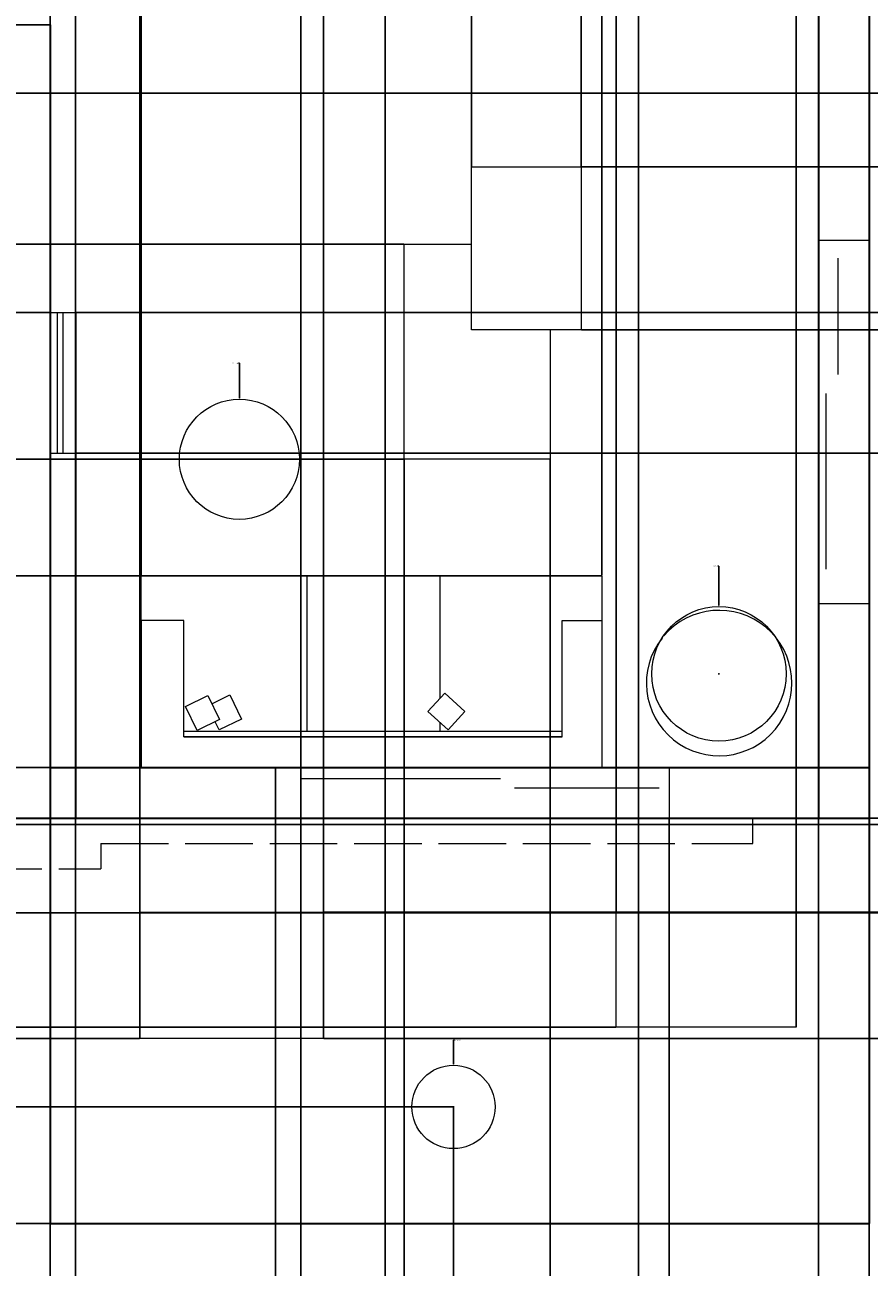
# Model space of a CAD drawing. Units: inches. Extents: x -47 to 496, y -43 to 706.
# Tile 3 of 6: x 209 to 359, y 123 to 344. Entities that reach past the tile are written whole.
import ezdxf

# ---------------------------------------------------------------- set-up
doc = ezdxf.new("R2010")
doc.units = ezdxf.units.IN
doc.linetypes.add('ACAD_ISO02W100', pattern=[15, 12, -3])
for name, color, linetype, lineweight in [('A-ANNO-DIMS', 2, 'Continuous', 18), ('A-ROOF-OVHD', 8, 'ACAD_ISO02W100', 18), ('FURNITURE', 3, 'Continuous', 18), ('WALL', 7, 'Continuous', 35), ('WINDOW', 1, 'Continuous', 18)]:
    doc.layers.add(name, color=color, linetype=linetype, lineweight=lineweight)
doc.styles.get("Standard").update_dxf_attribs({"font": 'arial.ttf'})
doc.dimstyles.get("Standard").update_dxf_attribs({"dimtxt": 0.18, "dimasz": 0.18, "dimexe": 0.18, "dimexo": 0.0625, "dimgap": 0.09, "dimtad": 0, "dimtih": 1, "dimtoh": 1, "dimdec": 4, "dimzin": 0, "dimdsep": 46, "dimtxsty": 'Standard', "dimcen": 0.09, "dimadec": 0, "dimazin": 0, "dimtfac": 1, "dimtdec": 4, "dimtofl": 0, "dimtmove": 0, "dimatfit": 3, "dimfxl": 1, "dimtolj": 1, "dimtzin": 0, "dimarcsym": 0})

# ---------------------------------------------------------------- blocks, each defined once
blk = doc.blocks.new('*D21')
at = {"layer": 'A-ANNO-DIMS', "color": 0, "lineweight": -2, "transparency": 16777216}
for p, q in [((213.95, 130.91), (213.95, -42.84)), ((359.45, 130.91), (359.45, -42.84)), ((214.13, -42.66), (286.32, -42.66)), ((359.27, -42.66), (287.09, -42.66))]:
    blk.add_line(p, q, dxfattribs=at)
at = {"layer": 'A-ANNO-DIMS', "color": 0, "transparency": 16777216}
for points in [[(214.13, -42.63), (214.13, -42.69), (213.95, -42.66)], [(359.27, -42.63), (359.27, -42.69), (359.45, -42.66)]]:
    blk.add_solid(points, dxfattribs=at)
at = {"layer": 'Defpoints', "color": 0, "transparency": 16777216}
for p in [(213.95, 130.97), (359.45, 130.97), (359.45, -42.66)]:
    blk.add_point(p, dxfattribs=at)
at = {"layer": 'A-ANNO-DIMS', "color": 0, "transparency": 16777216, "insert": (286.7, -42.66), "char_height": 0.18, "attachment_point": 5}
blk.add_mtext('\\A1;145.5', dxfattribs=at)
blk = doc.blocks.new('*D22')
at = {"layer": 'A-ANNO-DIMS', "color": 0, "lineweight": -2, "transparency": 16777216}
for p, q in [((229.88, 163.9), (229.88, 705.7)), ((230.06, 705.52), (245.73, 705.52)), ((262.33, 705.52), (246.66, 705.52)), ((262.51, 163.9), (262.51, 705.7))]:
    blk.add_line(p, q, dxfattribs=at)
at = {"layer": 'A-ANNO-DIMS', "color": 0, "transparency": 16777216}
for points in [[(230.06, 705.55), (230.06, 705.49), (229.88, 705.52)], [(262.33, 705.55), (262.33, 705.49), (262.51, 705.52)]]:
    blk.add_solid(points, dxfattribs=at)
at = {"layer": 'Defpoints', "color": 0, "transparency": 16777216}
for p in [(262.51, 705.52), (229.88, 163.83), (262.51, 163.83)]:
    blk.add_point(p, dxfattribs=at)
at = {"layer": 'A-ANNO-DIMS', "color": 0, "transparency": 16777216, "insert": (246.2, 705.52), "char_height": 0.18, "attachment_point": 5}
blk.add_mtext('\\A1;32.636', dxfattribs=at)
blk = doc.blocks.new('*D23')
at = {"layer": 'A-ANNO-DIMS', "color": 0, "lineweight": -2, "transparency": 16777216}
for p, q in [((262.58, 186.29), (496.14, 186.29)), ((495.96, 186.11), (495.96, 175.24)), ((495.96, 164.01), (495.96, 174.88)), ((262.58, 163.83), (496.14, 163.83))]:
    blk.add_line(p, q, dxfattribs=at)
at = {"layer": 'A-ANNO-DIMS', "color": 0, "transparency": 16777216}
for points in [[(495.93, 186.11), (495.99, 186.11), (495.96, 186.29)], [(495.93, 164.01), (495.99, 164.01), (495.96, 163.83)]]:
    blk.add_solid(points, dxfattribs=at)
at = {"layer": 'Defpoints', "color": 0, "transparency": 16777216}
for p in [(262.51, 186.29), (495.96, 186.29), (262.51, 163.83)]:
    blk.add_point(p, dxfattribs=at)
at = {"layer": 'A-ANNO-DIMS', "color": 0, "transparency": 16777216, "insert": (495.96, 175.06), "char_height": 0.18, "attachment_point": 5}
blk.add_mtext('\\A1;22.45', dxfattribs=at)
blk = doc.blocks.new('*D24')
at = {"layer": 'A-ANNO-DIMS', "color": 0, "lineweight": -2, "transparency": 16777216}
for p, q in [((314.53, 186.25), (314.53, 705.7)), ((314.71, 705.52), (330.12, 705.52)), ((346.32, 705.52), (330.91, 705.52)), ((346.5, 186.25), (346.5, 705.7))]:
    blk.add_line(p, q, dxfattribs=at)
at = {"layer": 'A-ANNO-DIMS', "color": 0, "transparency": 16777216}
for points in [[(314.71, 705.55), (314.71, 705.49), (314.53, 705.52)], [(346.32, 705.55), (346.32, 705.49), (346.5, 705.52)]]:
    blk.add_solid(points, dxfattribs=at)
at = {"layer": 'Defpoints', "color": 0, "transparency": 16777216}
for p in [(346.5, 705.52), (314.53, 186.18), (346.5, 186.18)]:
    blk.add_point(p, dxfattribs=at)
at = {"layer": 'A-ANNO-DIMS', "color": 0, "transparency": 16777216, "insert": (330.52, 705.52), "char_height": 0.18, "attachment_point": 5}
blk.add_mtext('\\A1;31.97', dxfattribs=at)
blk = doc.blocks.new('*D25')
at = {"layer": 'A-ANNO-DIMS', "color": 0, "lineweight": -2, "transparency": 16777216}
for p, q in [((314.47, 186.18), (-47.29, 186.18)), ((-47.11, 186), (-47.11, 176.21)), ((-47.11, 166.05), (-47.11, 175.84)), ((314.47, 165.87), (-47.29, 165.87))]:
    blk.add_line(p, q, dxfattribs=at)
at = {"layer": 'A-ANNO-DIMS', "color": 0, "transparency": 16777216}
for points in [[(-47.14, 186), (-47.08, 186), (-47.11, 186.18)], [(-47.14, 166.05), (-47.08, 166.05), (-47.11, 165.87)]]:
    blk.add_solid(points, dxfattribs=at)
at = {"layer": 'Defpoints', "color": 0, "transparency": 16777216}
for p in [(-47.11, 186.18), (314.53, 186.18), (314.53, 165.87)]:
    blk.add_point(p, dxfattribs=at)
at = {"layer": 'A-ANNO-DIMS', "color": 0, "transparency": 16777216, "insert": (-47.11, 176.03), "char_height": 0.18, "attachment_point": 5}
blk.add_mtext('\\A1;20.318', dxfattribs=at)
blk = doc.blocks.new('*D26')
at = {"layer": 'A-ANNO-DIMS', "color": 0, "lineweight": -2, "transparency": 16777216}
for p, q in [((213.95, 131.03), (213.95, 705.7)), ((214.13, 705.52), (221.46, 705.52)), ((229.7, 705.52), (222.37, 705.52)), ((229.88, 163.9), (229.88, 705.7))]:
    blk.add_line(p, q, dxfattribs=at)
at = {"layer": 'A-ANNO-DIMS', "color": 0, "transparency": 16777216}
for points in [[(214.13, 705.55), (214.13, 705.49), (213.95, 705.52)], [(229.7, 705.55), (229.7, 705.49), (229.88, 705.52)]]:
    blk.add_solid(points, dxfattribs=at)
at = {"layer": 'Defpoints', "color": 0, "transparency": 16777216}
for p in [(229.88, 705.52), (229.88, 163.83), (213.95, 130.97)]:
    blk.add_point(p, dxfattribs=at)
at = {"layer": 'A-ANNO-DIMS', "color": 0, "transparency": 16777216, "insert": (221.92, 705.52), "char_height": 0.18, "attachment_point": 5}
blk.add_mtext('\\A1;15.924', dxfattribs=at)
blk = doc.blocks.new('*D27')
at = {"layer": 'A-ANNO-DIMS', "color": 0, "lineweight": -2, "transparency": 16777216}
for p, q in [((229.82, 163.83), (-47.29, 163.83)), ((-47.11, 163.65), (-47.11, 147.58)), ((-47.11, 131.15), (-47.11, 147.22)), ((213.89, 130.97), (-47.29, 130.97))]:
    blk.add_line(p, q, dxfattribs=at)
at = {"layer": 'A-ANNO-DIMS', "color": 0, "transparency": 16777216}
for points in [[(-47.14, 163.65), (-47.08, 163.65), (-47.11, 163.83)], [(-47.14, 131.15), (-47.08, 131.15), (-47.11, 130.97)]]:
    blk.add_solid(points, dxfattribs=at)
at = {"layer": 'Defpoints', "color": 0, "transparency": 16777216}
for p in [(-47.11, 163.83), (229.88, 163.83), (213.95, 130.97)]:
    blk.add_point(p, dxfattribs=at)
at = {"layer": 'A-ANNO-DIMS', "color": 0, "transparency": 16777216, "insert": (-47.11, 147.4), "char_height": 0.18, "attachment_point": 5}
blk.add_mtext('\\A1;32.864', dxfattribs=at)
blk = doc.blocks.new('*D28')
at = {"layer": 'A-ANNO-DIMS', "color": 0, "lineweight": -2, "transparency": 16777216}
for p, q in [((346.5, 165.93), (346.5, 705.7)), ((346.68, 705.52), (352.52, 705.52)), ((359.27, 705.52), (353.43, 705.52)), ((359.45, 131.03), (359.45, 705.7))]:
    blk.add_line(p, q, dxfattribs=at)
at = {"layer": 'A-ANNO-DIMS', "color": 0, "transparency": 16777216}
for points in [[(346.68, 705.55), (346.68, 705.49), (346.5, 705.52)], [(359.27, 705.55), (359.27, 705.49), (359.45, 705.52)]]:
    blk.add_solid(points, dxfattribs=at)
at = {"layer": 'Defpoints', "color": 0, "transparency": 16777216}
for p in [(359.45, 705.52), (346.5, 165.87), (359.45, 130.97)]:
    blk.add_point(p, dxfattribs=at)
at = {"layer": 'A-ANNO-DIMS', "color": 0, "transparency": 16777216, "insert": (352.98, 705.52), "char_height": 0.18, "attachment_point": 5}
blk.add_mtext('\\A1;12.954', dxfattribs=at)
blk = doc.blocks.new('*D29')
at = {"layer": 'A-ANNO-DIMS', "color": 0, "lineweight": -2, "transparency": 16777216}
for p, q in [((359.52, 202.97), (496.14, 202.97)), ((495.96, 202.79), (495.96, 194.76)), ((495.96, 186.36), (495.96, 194.4)), ((346.56, 186.18), (496.14, 186.18))]:
    blk.add_line(p, q, dxfattribs=at)
at = {"layer": 'A-ANNO-DIMS', "color": 0, "transparency": 16777216}
for points in [[(495.93, 202.79), (495.99, 202.79), (495.96, 202.97)], [(495.93, 186.36), (495.99, 186.36), (495.96, 186.18)]]:
    blk.add_solid(points, dxfattribs=at)
at = {"layer": 'Defpoints', "color": 0, "transparency": 16777216}
for p in [(359.45, 202.97), (495.96, 202.97), (346.5, 186.18)]:
    blk.add_point(p, dxfattribs=at)
at = {"layer": 'A-ANNO-DIMS', "color": 0, "transparency": 16777216, "insert": (495.96, 194.58), "char_height": 0.18, "attachment_point": 5}
blk.add_mtext('\\A1;16.787', dxfattribs=at)
blk = doc.blocks.new('*D30')
at = {"layer": 'A-ANNO-DIMS', "color": 0, "lineweight": -2, "transparency": 16777216}
for p, q in [((285.61, 151.6), (285.61, -42.84)), ((213.95, 130.91), (213.95, -42.84)), ((214.13, -42.66), (249.39, -42.66)), ((285.43, -42.66), (250.18, -42.66))]:
    blk.add_line(p, q, dxfattribs=at)
at = {"layer": 'A-ANNO-DIMS', "color": 0, "transparency": 16777216}
for points in [[(214.13, -42.63), (214.13, -42.69), (213.95, -42.66)], [(285.43, -42.63), (285.43, -42.69), (285.61, -42.66)]]:
    blk.add_solid(points, dxfattribs=at)
at = {"layer": 'Defpoints', "color": 0, "transparency": 16777216}
for p in [(285.61, 151.67), (213.95, 130.97), (285.61, -42.66)]:
    blk.add_point(p, dxfattribs=at)
at = {"layer": 'A-ANNO-DIMS', "color": 0, "transparency": 16777216, "insert": (249.78, -42.66), "char_height": 0.18, "attachment_point": 5}
blk.add_mtext('\\A1;71.65', dxfattribs=at)
blk = doc.blocks.new('*D31')
at = {"layer": 'A-ANNO-DIMS', "color": 0, "lineweight": -2, "transparency": 16777216}
for p, q in [((285.55, 151.67), (-47.29, 151.67)), ((-47.11, 151.49), (-47.11, 141.5)), ((-47.11, 131.15), (-47.11, 141.14)), ((359.39, 130.97), (-47.29, 130.97))]:
    blk.add_line(p, q, dxfattribs=at)
at = {"layer": 'A-ANNO-DIMS', "color": 0, "transparency": 16777216}
for points in [[(-47.14, 151.49), (-47.08, 151.49), (-47.11, 151.67)], [(-47.14, 131.15), (-47.08, 131.15), (-47.11, 130.97)]]:
    blk.add_solid(points, dxfattribs=at)
at = {"layer": 'Defpoints', "color": 0, "transparency": 16777216}
for p in [(285.61, 151.67), (-47.11, 130.97), (359.45, 130.97)]:
    blk.add_point(p, dxfattribs=at)
at = {"layer": 'A-ANNO-DIMS', "color": 0, "transparency": 16777216, "insert": (-47.11, 141.32), "char_height": 0.18, "attachment_point": 5}
blk.add_mtext('\\A1;20.695', dxfattribs=at)
blk = doc.blocks.new('*D35')
at = {"layer": 'A-ANNO-DIMS', "color": 0, "lineweight": -2, "transparency": 16777216}
for p, q in [((218.45, 484.91), (218.45, -42.84)), ((350.45, 480.41), (350.45, -42.84)), ((218.63, -42.66), (284.18, -42.66)), ((350.27, -42.66), (284.73, -42.66))]:
    blk.add_line(p, q, dxfattribs=at)
at = {"layer": 'A-ANNO-DIMS', "color": 0, "transparency": 16777216}
for points in [[(218.63, -42.63), (218.63, -42.69), (218.45, -42.66)], [(350.27, -42.63), (350.27, -42.69), (350.45, -42.66)]]:
    blk.add_solid(points, dxfattribs=at)
at = {"layer": 'Defpoints', "color": 0, "transparency": 16777216}
for p in [(218.45, 484.97), (350.45, 480.47), (350.45, -42.66)]:
    blk.add_point(p, dxfattribs=at)
at = {"layer": 'A-ANNO-DIMS', "color": 0, "transparency": 16777216, "insert": (284.45, -42.66), "char_height": 0.18, "attachment_point": 5}
blk.add_mtext('\\A1;132', dxfattribs=at)
blk = doc.blocks.new('*D51')
at = {"layer": 'A-ANNO-DIMS', "color": 0, "lineweight": -2, "transparency": 16777216}
for p, q in [((218.45, 621.91), (218.45, -42.84)), ((258.46, 619.91), (258.46, -42.84)), ((218.63, -42.66), (238.08, -42.66)), ((258.28, -42.66), (238.84, -42.66))]:
    blk.add_line(p, q, dxfattribs=at)
at = {"layer": 'A-ANNO-DIMS', "color": 0, "transparency": 16777216}
for points in [[(218.63, -42.63), (218.63, -42.69), (218.45, -42.66)], [(258.28, -42.63), (258.28, -42.69), (258.46, -42.66)]]:
    blk.add_solid(points, dxfattribs=at)
at = {"layer": 'Defpoints', "color": 0, "transparency": 16777216}
for p in [(218.45, 621.97), (258.46, 619.97), (258.46, -42.66)]:
    blk.add_point(p, dxfattribs=at)
at = {"layer": 'A-ANNO-DIMS', "color": 0, "transparency": 16777216, "insert": (238.46, -42.66), "char_height": 0.18, "attachment_point": 5}
blk.add_mtext('\\A1;40.01', dxfattribs=at)
blk = doc.blocks.new('*D54')
at = {"layer": 'A-ANNO-DIMS', "color": 0, "lineweight": -2, "transparency": 16777216}
for p, q in [((273.48, 348.41), (273.48, -42.84)), ((350.45, 348.41), (350.45, -42.84)), ((273.66, -42.66), (311.57, -42.66)), ((350.27, -42.66), (312.36, -42.66))]:
    blk.add_line(p, q, dxfattribs=at)
at = {"layer": 'A-ANNO-DIMS', "color": 0, "transparency": 16777216}
for points in [[(273.66, -42.63), (273.66, -42.69), (273.48, -42.66)], [(350.27, -42.63), (350.27, -42.69), (350.45, -42.66)]]:
    blk.add_solid(points, dxfattribs=at)
at = {"layer": 'Defpoints', "color": 0, "transparency": 16777216}
for p in [(273.48, 348.47), (350.45, 348.47), (350.45, -42.66)]:
    blk.add_point(p, dxfattribs=at)
at = {"layer": 'A-ANNO-DIMS', "color": 0, "transparency": 16777216, "insert": (311.97, -42.66), "char_height": 0.18, "attachment_point": 5}
blk.add_mtext('\\A1;76.97', dxfattribs=at)
blk = doc.blocks.new('*D59')
at = {"layer": 'A-ANNO-DIMS', "color": 0, "lineweight": -2, "transparency": 16777216}
for p, q in [((318.48, 390.41), (318.48, -42.84)), ((350.45, 390.41), (350.45, -42.84)), ((318.66, -42.66), (334, -42.66)), ((350.27, -42.66), (334.93, -42.66))]:
    blk.add_line(p, q, dxfattribs=at)
at = {"layer": 'A-ANNO-DIMS', "color": 0, "transparency": 16777216}
for points in [[(318.66, -42.63), (318.66, -42.69), (318.48, -42.66)], [(350.27, -42.63), (350.27, -42.69), (350.45, -42.66)]]:
    blk.add_solid(points, dxfattribs=at)
at = {"layer": 'Defpoints', "color": 0, "transparency": 16777216}
for p in [(318.48, 390.47), (350.45, 390.47), (350.45, -42.66)]:
    blk.add_point(p, dxfattribs=at)
at = {"layer": 'A-ANNO-DIMS', "color": 0, "transparency": 16777216, "insert": (334.47, -42.66), "char_height": 0.18, "attachment_point": 5}
blk.add_mtext('\\A1;31.975', dxfattribs=at)
blk = doc.blocks.new('*D64')
at = {"layer": 'A-ANNO-DIMS', "color": 0, "lineweight": -2, "transparency": 16777216}
for p, q in [((158.02, 343.91), (158.02, -42.84)), ((218.45, 343.91), (218.45, -42.84)), ((158.2, -42.66), (187.84, -42.66)), ((218.27, -42.66), (188.63, -42.66))]:
    blk.add_line(p, q, dxfattribs=at)
at = {"layer": 'A-ANNO-DIMS', "color": 0, "transparency": 16777216}
for points in [[(158.2, -42.63), (158.2, -42.69), (158.02, -42.66)], [(218.27, -42.63), (218.27, -42.69), (218.45, -42.66)]]:
    blk.add_solid(points, dxfattribs=at)
at = {"layer": 'Defpoints', "color": 0, "transparency": 16777216}
for p in [(158.02, 343.97), (218.45, 343.97), (218.45, -42.66)]:
    blk.add_point(p, dxfattribs=at)
at = {"layer": 'A-ANNO-DIMS', "color": 0, "transparency": 16777216, "insert": (188.24, -42.66), "char_height": 0.18, "attachment_point": 5}
blk.add_mtext('\\A1;60.43', dxfattribs=at)
blk = doc.blocks.new('*D65')
at = {"layer": 'A-ANNO-DIMS', "color": 0, "lineweight": -2, "transparency": 16777216}
for p, q in [((218.45, 348.41), (218.45, -42.84)), ((273.48, 348.41), (273.48, -42.84)), ((218.63, -42.66), (245.57, -42.66)), ((273.3, -42.66), (246.36, -42.66))]:
    blk.add_line(p, q, dxfattribs=at)
at = {"layer": 'A-ANNO-DIMS', "color": 0, "transparency": 16777216}
for points in [[(218.63, -42.63), (218.63, -42.69), (218.45, -42.66)], [(273.3, -42.63), (273.3, -42.69), (273.48, -42.66)]]:
    blk.add_solid(points, dxfattribs=at)
at = {"layer": 'Defpoints', "color": 0, "transparency": 16777216}
for p in [(218.45, 348.47), (273.48, 348.47), (273.48, -42.66)]:
    blk.add_point(p, dxfattribs=at)
at = {"layer": 'A-ANNO-DIMS', "color": 0, "transparency": 16777216, "insert": (245.97, -42.66), "char_height": 0.18, "attachment_point": 5}
blk.add_mtext('\\A1;55.03', dxfattribs=at)
blk = doc.blocks.new('*D73')
at = {"layer": 'A-ANNO-DIMS', "color": 0, "lineweight": -2, "transparency": 16777216}
for p, q in [((213.95, 211.91), (213.95, -42.84)), ((195.95, 202.91), (195.95, -42.84)), ((196.13, -42.66), (204.74, -42.66)), ((213.77, -42.66), (205.17, -42.66))]:
    blk.add_line(p, q, dxfattribs=at)
at = {"layer": 'A-ANNO-DIMS', "color": 0, "transparency": 16777216}
for points in [[(196.13, -42.63), (196.13, -42.69), (195.95, -42.66)], [(213.77, -42.63), (213.77, -42.69), (213.95, -42.66)]]:
    blk.add_solid(points, dxfattribs=at)
at = {"layer": 'Defpoints', "color": 0, "transparency": 16777216}
for p in [(213.95, 211.97), (195.95, 202.97), (213.95, -42.66)]:
    blk.add_point(p, dxfattribs=at)
at = {"layer": 'A-ANNO-DIMS', "color": 0, "transparency": 16777216, "insert": (204.95, -42.66), "char_height": 0.18, "attachment_point": 5}
blk.add_mtext('\\A1;18', dxfattribs=at)
blk = doc.blocks.new('*D74')
at = {"layer": 'A-ANNO-DIMS', "color": 0, "lineweight": -2, "transparency": 16777216}
for p, q in [((213.95, 211.91), (213.95, -42.84)), ((254, 211.91), (254, -42.84)), ((214.13, -42.66), (233.58, -42.66)), ((253.82, -42.66), (234.38, -42.66))]:
    blk.add_line(p, q, dxfattribs=at)
at = {"layer": 'A-ANNO-DIMS', "color": 0, "transparency": 16777216}
for points in [[(214.13, -42.63), (214.13, -42.69), (213.95, -42.66)], [(253.82, -42.63), (253.82, -42.69), (254, -42.66)]]:
    blk.add_solid(points, dxfattribs=at)
at = {"layer": 'Defpoints', "color": 0, "transparency": 16777216}
for p in [(213.95, 211.97), (254, 211.97), (254, -42.66)]:
    blk.add_point(p, dxfattribs=at)
at = {"layer": 'A-ANNO-DIMS', "color": 0, "transparency": 16777216, "insert": (233.98, -42.66), "char_height": 0.18, "attachment_point": 5}
blk.add_mtext('\\A1;40.05', dxfattribs=at)
blk = doc.blocks.new('*D75')
at = {"layer": 'A-ANNO-DIMS', "color": 0, "lineweight": -2, "transparency": 16777216}
for p, q in [((254, 202.91), (254, -42.84)), ((323.91, 202.91), (323.91, -42.84)), ((254.18, -42.66), (288.58, -42.66)), ((323.73, -42.66), (289.33, -42.66))]:
    blk.add_line(p, q, dxfattribs=at)
at = {"layer": 'A-ANNO-DIMS', "color": 0, "transparency": 16777216}
for points in [[(254.18, -42.63), (254.18, -42.69), (254, -42.66)], [(323.73, -42.63), (323.73, -42.69), (323.91, -42.66)]]:
    blk.add_solid(points, dxfattribs=at)
at = {"layer": 'Defpoints', "color": 0, "transparency": 16777216}
for p in [(254, 202.97), (323.91, 202.97), (323.91, -42.66)]:
    blk.add_point(p, dxfattribs=at)
at = {"layer": 'A-ANNO-DIMS', "color": 0, "transparency": 16777216, "insert": (288.96, -42.66), "char_height": 0.18, "attachment_point": 5}
blk.add_mtext('\\A1;69.91', dxfattribs=at)
blk = doc.blocks.new('*D78')
at = {"layer": 'A-ANNO-DIMS', "color": 0, "lineweight": -2, "transparency": 16777216}
for p, q in [((230.13, 246.14), (230.13, 705.7)), ((230.31, 705.52), (270.64, 705.52)), ((311.77, 705.52), (271.43, 705.52)), ((311.95, 246.14), (311.95, 705.7))]:
    blk.add_line(p, q, dxfattribs=at)
at = {"layer": 'A-ANNO-DIMS', "color": 0, "transparency": 16777216}
for points in [[(230.31, 705.55), (230.31, 705.49), (230.13, 705.52)], [(311.77, 705.55), (311.77, 705.49), (311.95, 705.52)]]:
    blk.add_solid(points, dxfattribs=at)
at = {"layer": 'Defpoints', "color": 0, "transparency": 16777216}
for p in [(311.95, 705.52), (230.13, 246.07), (311.95, 246.07)]:
    blk.add_point(p, dxfattribs=at)
at = {"layer": 'A-ANNO-DIMS', "color": 0, "transparency": 16777216, "insert": (271.04, 705.52), "char_height": 0.18, "attachment_point": 5}
blk.add_mtext('\\A1;81.82', dxfattribs=at)
blk = doc.blocks.new('*D79')
at = {"layer": 'A-ANNO-DIMS', "color": 0, "lineweight": -2, "transparency": 16777216}
for p, q in [((311.88, 246.07), (-47.29, 246.07)), ((-47.11, 245.89), (-47.11, 229.2)), ((-47.11, 212.15), (-47.11, 228.84)), ((311.88, 211.97), (-47.29, 211.97))]:
    blk.add_line(p, q, dxfattribs=at)
at = {"layer": 'A-ANNO-DIMS', "color": 0, "transparency": 16777216}
for points in [[(-47.14, 245.89), (-47.08, 245.89), (-47.11, 246.07)], [(-47.14, 212.15), (-47.08, 212.15), (-47.11, 211.97)]]:
    blk.add_solid(points, dxfattribs=at)
at = {"layer": 'Defpoints', "color": 0, "transparency": 16777216}
for p in [(-47.11, 246.07), (311.95, 246.07), (311.95, 211.97)]:
    blk.add_point(p, dxfattribs=at)
at = {"layer": 'A-ANNO-DIMS', "color": 0, "transparency": 16777216, "insert": (-47.11, 229.02), "char_height": 0.18, "attachment_point": 5}
blk.add_mtext('\\A1;34.103', dxfattribs=at)
blk = doc.blocks.new('*D80')
at = {"layer": 'A-ANNO-DIMS', "color": 0, "lineweight": -2, "transparency": 16777216}
for p, q in [((218.52, 292.83), (496.14, 292.83)), ((495.96, 292.65), (495.96, 280.53)), ((495.96, 268.06), (495.96, 280.17)), ((218.52, 267.88), (496.14, 267.88))]:
    blk.add_line(p, q, dxfattribs=at)
at = {"layer": 'A-ANNO-DIMS', "color": 0, "transparency": 16777216}
for points in [[(495.93, 292.65), (495.99, 292.65), (495.96, 292.83)], [(495.93, 268.06), (495.99, 268.06), (495.96, 267.88)]]:
    blk.add_solid(points, dxfattribs=at)
at = {"layer": 'Defpoints', "color": 0, "transparency": 16777216}
for p in [(218.45, 292.83), (495.96, 292.83), (218.45, 267.88)]:
    blk.add_point(p, dxfattribs=at)
at = {"layer": 'A-ANNO-DIMS', "color": 0, "transparency": 16777216, "insert": (495.96, 280.35), "char_height": 0.18, "attachment_point": 5}
blk.add_mtext('\\A1;24.946', dxfattribs=at)
blk = doc.blocks.new('*D81')
at = {"layer": 'A-ANNO-DIMS', "color": 0, "lineweight": -2, "transparency": 16777216}
for p, q in [((213.89, 343.97), (-47.29, 343.97)), ((-47.11, 343.79), (-47.11, 318.58)), ((-47.11, 293.01), (-47.11, 318.22)), ((213.89, 292.83), (-47.29, 292.83))]:
    blk.add_line(p, q, dxfattribs=at)
at = {"layer": 'A-ANNO-DIMS', "color": 0, "transparency": 16777216}
for points in [[(-47.14, 343.79), (-47.08, 343.79), (-47.11, 343.97)], [(-47.14, 293.01), (-47.08, 293.01), (-47.11, 292.83)]]:
    blk.add_solid(points, dxfattribs=at)
at = {"layer": 'Defpoints', "color": 0, "transparency": 16777216}
for p in [(-47.11, 343.97), (213.95, 343.97), (213.95, 292.83)]:
    blk.add_point(p, dxfattribs=at)
at = {"layer": 'A-ANNO-DIMS', "color": 0, "transparency": 16777216, "insert": (-47.11, 318.4), "char_height": 0.18, "attachment_point": 5}
blk.add_mtext('\\A1;51.15', dxfattribs=at)
blk = doc.blocks.new('*D82')
at = {"layer": 'A-ANNO-DIMS', "color": 0, "lineweight": -2, "transparency": 16777216}
for p, q in [((108.88, 331.8), (496.14, 331.8)), ((495.96, 331.62), (495.96, 267)), ((495.96, 202.02), (495.96, 266.64)), ((131.48, 201.84), (496.14, 201.84))]:
    blk.add_line(p, q, dxfattribs=at)
at = {"layer": 'A-ANNO-DIMS', "color": 0, "transparency": 16777216}
for points in [[(495.93, 331.62), (495.99, 331.62), (495.96, 331.8)], [(495.93, 202.02), (495.99, 202.02), (495.96, 201.84)]]:
    blk.add_solid(points, dxfattribs=at)
at = {"layer": 'Defpoints', "color": 0, "transparency": 16777216}
for p in [(108.82, 331.8), (131.41, 201.84), (495.96, 201.84)]:
    blk.add_point(p, dxfattribs=at)
at = {"layer": 'A-ANNO-DIMS', "color": 0, "transparency": 16777216, "insert": (495.96, 266.82), "char_height": 0.18, "attachment_point": 5}
blk.add_mtext('\\A1;129.95', dxfattribs=at)
blk = doc.blocks.new('*D84')
at = {"layer": 'A-ANNO-DIMS', "color": 0, "lineweight": -2, "transparency": 16777216}
for p, q in [((276.84, 266.72), (276.84, -42.84)), ((302.79, 266.72), (302.79, -42.84)), ((277.02, -42.66), (289.42, -42.66)), ((302.61, -42.66), (290.21, -42.66))]:
    blk.add_line(p, q, dxfattribs=at)
at = {"layer": 'A-ANNO-DIMS', "color": 0, "transparency": 16777216}
for points in [[(277.02, -42.63), (277.02, -42.69), (276.84, -42.66)], [(302.61, -42.63), (302.61, -42.69), (302.79, -42.66)]]:
    blk.add_solid(points, dxfattribs=at)
at = {"layer": 'Defpoints', "color": 0, "transparency": 16777216}
for p in [(276.84, 266.78), (302.79, 266.78), (302.79, -42.66)]:
    blk.add_point(p, dxfattribs=at)
at = {"layer": 'A-ANNO-DIMS', "color": 0, "transparency": 16777216, "insert": (289.82, -42.66), "char_height": 0.18, "attachment_point": 5}
blk.add_mtext('\\A1;25.95', dxfattribs=at)
blk = doc.blocks.new('*D85')
at = {"layer": 'A-ANNO-DIMS', "color": 0, "lineweight": -2, "transparency": 16777216}
for p, q in [((276.78, 305.01), (-47.29, 305.01)), ((-47.11, 304.83), (-47.11, 286.08)), ((-47.11, 266.96), (-47.11, 285.71)), ((276.78, 266.78), (-47.29, 266.78))]:
    blk.add_line(p, q, dxfattribs=at)
at = {"layer": 'A-ANNO-DIMS', "color": 0, "transparency": 16777216}
for points in [[(-47.14, 304.83), (-47.08, 304.83), (-47.11, 305.01)], [(-47.14, 266.96), (-47.08, 266.96), (-47.11, 266.78)]]:
    blk.add_solid(points, dxfattribs=at)
at = {"layer": 'Defpoints', "color": 0, "transparency": 16777216}
for p in [(-47.11, 305.01), (276.84, 305.01), (276.84, 266.78)]:
    blk.add_point(p, dxfattribs=at)
at = {"layer": 'A-ANNO-DIMS', "color": 0, "transparency": 16777216, "insert": (-47.11, 285.9), "char_height": 0.18, "attachment_point": 5}
blk.add_mtext('\\A1;38.22', dxfattribs=at)
blk = doc.blocks.new('*D86')
at = {"layer": 'A-ANNO-DIMS', "color": 0, "lineweight": -2, "transparency": 16777216}
for p, q in [((288.82, 318.79), (288.82, 705.7)), ((289, 705.52), (298.16, 705.52)), ((308.09, 705.52), (298.93, 705.52)), ((308.27, 318.79), (308.27, 705.7))]:
    blk.add_line(p, q, dxfattribs=at)
at = {"layer": 'A-ANNO-DIMS', "color": 0, "transparency": 16777216}
for points in [[(289, 705.55), (289, 705.49), (288.82, 705.52)], [(308.09, 705.55), (308.09, 705.49), (308.27, 705.52)]]:
    blk.add_solid(points, dxfattribs=at)
at = {"layer": 'Defpoints', "color": 0, "transparency": 16777216}
for p in [(308.27, 705.52), (288.82, 318.72), (308.27, 318.72)]:
    blk.add_point(p, dxfattribs=at)
at = {"layer": 'A-ANNO-DIMS', "color": 0, "transparency": 16777216, "insert": (298.54, 705.52), "char_height": 0.18, "attachment_point": 5}
blk.add_mtext('\\A1;19.45', dxfattribs=at)
blk = doc.blocks.new('*D87')
at = {"layer": 'A-ANNO-DIMS', "color": 0, "lineweight": -2, "transparency": 16777216}
for p, q in [((308.33, 318.72), (496.14, 318.72)), ((495.96, 318.54), (495.96, 304.44)), ((495.96, 289.97), (495.96, 304.07)), ((308.33, 289.79), (496.14, 289.79))]:
    blk.add_line(p, q, dxfattribs=at)
at = {"layer": 'A-ANNO-DIMS', "color": 0, "transparency": 16777216}
for points in [[(495.93, 318.54), (495.99, 318.54), (495.96, 318.72)], [(495.93, 289.97), (495.99, 289.97), (495.96, 289.79)]]:
    blk.add_solid(points, dxfattribs=at)
at = {"layer": 'Defpoints', "color": 0, "transparency": 16777216}
for p in [(308.27, 318.72), (495.96, 318.72), (308.27, 289.79)]:
    blk.add_point(p, dxfattribs=at)
at = {"layer": 'A-ANNO-DIMS', "color": 0, "transparency": 16777216, "insert": (495.96, 304.26), "char_height": 0.18, "attachment_point": 5}
blk.add_mtext('\\A1;28.94', dxfattribs=at)
blk = doc.blocks.new('*D88')
at = {"layer": 'A-ANNO-DIMS', "color": 0, "lineweight": -2, "transparency": 16777216}
for p, q in [((285.79, 163.51), (285.61, 163.51)), ((285.61, 163.51), (285.61, 159.25)), ((285.52, 151.67), (285.7, 151.67)), ((285.61, 151.58), (285.61, 151.76))]:
    blk.add_line(p, q, dxfattribs=at)
at = {"layer": 'A-ANNO-DIMS', "color": 0, "transparency": 16777216}
blk.add_solid([(285.58, 159.25), (285.64, 159.25), (285.61, 159.07)], dxfattribs=at)
at = {"layer": 'Defpoints', "color": 0, "transparency": 16777216}
for p in [(285.61, 159.07), (285.61, 144.26)]:
    blk.add_point(p, dxfattribs=at)
at = {"layer": 'A-ANNO-DIMS', "color": 0, "transparency": 16777216, "insert": (286.35, 163.51), "char_height": 0.18, "attachment_point": 5}
blk.add_mtext('\\A1;∅14.807', dxfattribs=at)
blk = doc.blocks.new('*D90')
at = {"layer": 'A-ANNO-DIMS', "color": 0, "lineweight": -2, "transparency": 16777216}
for p, q in [((332.59, 247.76), (332.77, 247.76)), ((332.77, 247.76), (332.77, 240.76)), ((332.68, 228.63), (332.86, 228.63)), ((332.77, 228.54), (332.77, 228.72))]:
    blk.add_line(p, q, dxfattribs=at)
at = {"layer": 'A-ANNO-DIMS', "color": 0, "transparency": 16777216}
blk.add_solid([(332.8, 240.76), (332.74, 240.76), (332.77, 240.58)], dxfattribs=at)
at = {"layer": 'Defpoints', "color": 0, "transparency": 16777216}
for p in [(332.77, 240.58), (332.77, 216.68)]:
    blk.add_point(p, dxfattribs=at)
at = {"layer": 'A-ANNO-DIMS', "color": 0, "transparency": 16777216, "insert": (332.12, 247.76), "char_height": 0.18, "attachment_point": 5}
blk.add_mtext('\\A1;∅23.91', dxfattribs=at)
blk = doc.blocks.new('*D91')
at = {"layer": 'A-ANNO-DIMS', "color": 0, "lineweight": -2, "transparency": 16777216}
for p, q in [((247.4, 283.85), (247.58, 283.85)), ((247.58, 283.85), (247.58, 277.62)), ((247.49, 266.77), (247.67, 266.77)), ((247.58, 266.68), (247.58, 266.86))]:
    blk.add_line(p, q, dxfattribs=at)
at = {"layer": 'A-ANNO-DIMS', "color": 0, "transparency": 16777216}
blk.add_solid([(247.61, 277.62), (247.55, 277.62), (247.58, 277.44)], dxfattribs=at)
at = {"layer": 'Defpoints', "color": 0, "transparency": 16777216}
for p in [(247.58, 277.44), (247.58, 256.09)]:
    blk.add_point(p, dxfattribs=at)
at = {"layer": 'A-ANNO-DIMS', "color": 0, "transparency": 16777216, "insert": (246.84, 283.85), "char_height": 0.18, "attachment_point": 5}
blk.add_mtext('\\A1;∅21.354', dxfattribs=at)

msp = doc.modelspace()

# ---------------------------------------------------------------- linework, layer by layer
at = {"layer": 'A-ROOF-OVHD'}
for p, q in [((338.7999, 198.4711), (338.7999, 202.9711)), ((222.9545, 198.4711), (338.7999, 198.4711)), ((222.9545, 198.4711), (222.9545, 193.9711)), ((170.4932, 193.9711), (222.9545, 193.9711))]:
    msp.add_line(p, q, dxfattribs=at)
at = {"layer": 'FURNITURE'}
for p, q in [((259.5909, 218.421), (259.5909, 246.0745)), ((283.2401, 224.2901), (283.2401, 246.0745)), ((283.2401, 218.421), (283.2401, 219.9332))]:
    msp.add_line(p, q, dxfattribs=at)
for points in [[(288.8165, 318.7246), (308.2664, 318.7246), (308.2664, 289.7875), (288.8165, 289.7875)], [(237.9876, 222.8252), (241.971, 224.7682), (244.0536, 220.4987), (240.0702, 218.5557)], [(284.6398, 218.6567), (281.0709, 221.9114), (284.0659, 225.1956), (287.6349, 221.9409)], [(229.8783, 186.2855), (262.5138, 186.2855), (262.5138, 163.8346), (229.8783, 163.8346)], [(314.5329, 186.184), (346.5, 186.184), (346.5, 165.8664), (314.5329, 165.8664)]]:
    msp.add_lwpolyline(points, close=True, dxfattribs=at)
for points in [[(302.7925, 289.7875), (302.7925, 266.7848), (276.8411, 266.7848), (276.8411, 305.006), (288.8165, 305.006)], [(230.1291, 217.421), (230.1291, 246.0745), (311.9452, 246.0745), (311.9452, 217.421)], [(237.7272, 217.421), (237.7272, 238.1389), (230.1291, 238.1389), (230.1291, 211.9711), (237.7272, 211.9711)], [(304.9418, 217.421), (304.9418, 238.1389), (311.9452, 238.1389), (311.9452, 211.9711), (304.9418, 211.9711)], [(242.6823, 223.31), (245.8862, 224.8728), (247.9687, 220.6032), (243.9853, 218.6603), (243.2741, 220.1185)], [(311.9452, 217.421), (311.9452, 211.9711), (230.1291, 211.9711), (230.1291, 217.421)], [(237.7272, 218.421), (304.9418, 218.421)], [(237.7272, 217.421), (304.9418, 217.421)], [(304.9418, 217.421), (237.7272, 217.421)]]:
    msp.add_lwpolyline(points, dxfattribs=at)
for centre, radius in [((247.5772, 266.7661), 10.6769), ((332.7731, 228.6297), 11.9539), ((285.6085, 151.6661), 7.4034)]:
    msp.add_circle(centre, radius, dxfattribs=at)
msp.add_arc((332.8044, 226.9925), 12.9245, 141.764596, 139.573954, dxfattribs=at)
at = {"layer": 'WALL'}
for p, q in [((350.4545, 635.4711), (350.4545, 202.9711)), ((359.4545, 635.4711), (359.4545, 130.9711)), ((213.9545, 343.9711), (213.9545, 130.9711)), ((218.4545, 292.8257), (218.4545, 202.9711)), ((213.9545, 211.9711), (359.4545, 211.9711)), ((195.9545, 202.9711), (359.4545, 202.9711)), ((213.9545, 130.9711), (359.4545, 130.9711))]:
    msp.add_line(p, q, dxfattribs=at)
at = {"layer": 'WINDOW'}
for p, q in [((350.4545, 305.6843), (359.4545, 305.6843)), ((353.9691, 281.8522), (353.9691, 302.4765)), ((213.9545, 292.8257), (218.4545, 292.8257)), ((215.1987, 292.8257), (215.1987, 267.8798)), ((216.2045, 292.8257), (216.2045, 267.8798)), ((351.7782, 278.4445), (351.7782, 247.253)), ((213.9545, 267.8798), (218.4545, 267.8798)), ((350.4545, 241.1376), (359.4545, 241.1376)), ((254.0024, 211.9711), (254.0024, 202.9711)), ((323.9122, 211.9711), (323.9122, 202.9711)), ((258.6824, 210.0344), (293.9852, 210.0344)), ((296.4181, 208.3979), (322.1258, 208.3979))]:
    msp.add_line(p, q, dxfattribs=at)

# ---------------------------------------------------------------- dimensions: what is measured, and where the dimension line sits
at = {"layer": 'A-ANNO-DIMS'}
for base, p1, p2, override, picture, middle in [((229.8783, 705.5211), (213.9545, 130.9711), (229.8783, 163.8346), {"dimdec": 3, "dimlfac": 1, "dimrnd": 0, "dimzin": 0, "dimdsep": 46, "dimlunit": 2}, '*D26', (221.9164, 705.5211)), ((262.51385, 705.52106), (229.87829, 163.83464), (262.51385, 163.83464), {"dimdec": 3, "dimlfac": 1, "dimrnd": 0, "dimzin": 0, "dimdsep": 46, "dimlunit": 2}, '*D22', (246.19607, 705.52106)), ((311.9452, 705.5211), (230.1291, 246.0745), (311.9452, 246.0745), {"dimdec": 2, "dimlfac": 1, "dimrnd": 0, "dimzin": 0, "dimdsep": 46, "dimlunit": 2}, '*D78', (271.0372, 705.5211)), ((308.2664, 705.5211), (288.8165, 318.7246), (308.2664, 318.7246), {"dimdec": 2, "dimlfac": 1, "dimrnd": 0, "dimzin": 0, "dimdsep": 46, "dimlunit": 2}, '*D86', (298.5415, 705.5211)), ((346.5, 705.5211), (314.5329, 186.184), (346.5, 186.184), {"dimdec": 2, "dimlfac": 1, "dimrnd": 0, "dimzin": 0, "dimdsep": 46, "dimlunit": 2}, '*D24', (330.5165, 705.5211)), ((359.45448, 705.52106), (346.5, 165.86638), (359.45448, 130.97106), {"dimdec": 3, "dimlfac": 1, "dimrnd": 0, "dimzin": 0, "dimdsep": 46, "dimlunit": 2}, '*D28', (352.97724, 705.52106)), ((258.4633, -42.6632), (218.4545, 621.9711), (258.4633, 619.9711), {"dimdec": 2, "dimlfac": 1, "dimrnd": 0, "dimzin": 0, "dimdsep": 46, "dimlunit": 2}, '*D51', (238.4589, -42.6632)), ((350.4545, -42.6632), (218.4545, 484.9711), (350.4545, 480.4711), {"dimdec": 0, "dimlfac": 1, "dimrnd": 0, "dimzin": 0, "dimdsep": 46, "dimlunit": 2}, '*D35', (284.4545, -42.6632)), ((350.4545, -42.6632), (318.4798, 390.4711), (350.4545, 390.4711), {"dimdec": 3, "dimlfac": 1, "dimrnd": 0, "dimzin": 0, "dimdsep": 46, "dimlunit": 2}, '*D59', (334.4671, -42.6632)), ((273.4798, -42.6632), (218.4545, 348.4711), (273.4798, 348.4711), {"dimdec": 2, "dimlfac": 1, "dimrnd": 0, "dimzin": 0, "dimdsep": 46, "dimlunit": 2}, '*D65', (245.9671, -42.6632)), ((350.4545, -42.6632), (273.4798, 348.4711), (350.4545, 348.4711), {"dimdec": 2, "dimlfac": 1, "dimrnd": 0, "dimzin": 0, "dimdsep": 46, "dimlunit": 2}, '*D54', (311.9671, -42.6632)), ((218.4545, -42.6632), (158.0229, 343.9711), (218.4545, 343.9711), {"dimdec": 2, "dimlfac": 1, "dimrnd": 0, "dimzin": 0, "dimdsep": 46, "dimlunit": 2}, '*D64', (188.2387, -42.6632)), ((302.7925, -42.6632), (276.8411, 266.7848), (302.7925, 266.7848), {"dimdec": 2, "dimlfac": 1, "dimrnd": 0, "dimzin": 0, "dimdsep": 46, "dimlunit": 2}, '*D84', (289.8168, -42.6632)), ((213.9545, -42.6632), (195.9545, 202.9711), (213.9545, 211.9711), {"dimdec": 0, "dimlfac": 1, "dimrnd": 0, "dimzin": 0, "dimdsep": 46, "dimlunit": 2}, '*D73', (204.9545, -42.6632)), ((254.0024, -42.6632), (213.9545, 211.9711), (254.0024, 211.9711), {"dimdec": 2, "dimlfac": 1, "dimrnd": 0, "dimzin": 0, "dimdsep": 46, "dimlunit": 2}, '*D74', (233.9785, -42.6632)), ((323.9122, -42.6632), (254.0024, 202.9711), (323.9122, 202.9711), {"dimdec": 2, "dimlfac": 1, "dimrnd": 0, "dimzin": 0, "dimdsep": 46, "dimlunit": 2}, '*D75', (288.9573, -42.6632)), ((285.6085, -42.6632), (213.9545, 130.9711), (285.6085, 151.6661), {"dimdec": 2, "dimlfac": 1, "dimrnd": 0, "dimzin": 0, "dimdsep": 46, "dimlunit": 2}, '*D30', (249.7815, -42.6632)), ((359.4545, -42.6632), (213.9545, 130.9711), (359.4545, 130.9711), {"dimdec": 1, "dimlfac": 1, "dimrnd": 0, "dimzin": 0, "dimdsep": 46, "dimlunit": 2}, '*D21', (286.7045, -42.6632))]:
    dim = msp.add_linear_dim(base=base, p1=p1, p2=p2, dimstyle='Standard', override=override, dxfattribs=at)
    dim.commit()
    dim.dimension.update_dxf_attribs({"geometry": picture, "text_midpoint": middle})
for base, p1, p2, override, picture, middle in [((-47.1058, 343.9711), (213.9545, 292.8257), (213.9545, 343.9711), {"dimdec": 2, "dimlfac": 1, "dimrnd": 0, "dimzin": 0, "dimdsep": 46, "dimlunit": 2}, '*D81', (-47.1058, 318.3984)), ((495.9572, 201.8438), (108.8164, 331.7986), (131.4128, 201.8438), {"dimdec": 2, "dimlfac": 1, "dimrnd": 0, "dimzin": 0, "dimdsep": 46, "dimlunit": 2}, '*D82', (495.9572, 266.8212)), ((495.9572, 318.7246), (308.2664, 289.7875), (308.2664, 318.7246), {"dimdec": 2, "dimlfac": 1, "dimrnd": 0, "dimzin": 0, "dimdsep": 46, "dimlunit": 2}, '*D87', (495.9572, 304.2561)), ((-47.1058, 305.006), (276.8411, 266.7848), (276.8411, 305.006), {"dimdec": 2, "dimlfac": 1, "dimrnd": 0, "dimzin": 0, "dimdsep": 46, "dimlunit": 2}, '*D85', (-47.1058, 285.8954)), ((495.9572, 292.8257), (218.4545, 267.8798), (218.4545, 292.8257), {"dimdec": 3, "dimlfac": 1, "dimrnd": 0, "dimzin": 0, "dimdsep": 46, "dimlunit": 2}, '*D80', (495.9572, 280.3528)), ((-47.1058, 246.0745), (311.9452, 211.9711), (311.9452, 246.0745), {"dimdec": 3, "dimlfac": 1, "dimrnd": 0, "dimzin": 0, "dimdsep": 46, "dimlunit": 2}, '*D79', (-47.1058, 229.0228)), ((495.9572, 202.9711), (346.5, 186.184), (359.4545, 202.9711), {"dimdec": 3, "dimlfac": 1, "dimrnd": 0, "dimzin": 0, "dimdsep": 46, "dimlunit": 2}, '*D29', (495.9572, 194.5775)), ((-47.1058, 186.184), (314.5329, 165.8664), (314.5329, 186.184), {"dimdec": 3, "dimlfac": 1, "dimrnd": 0, "dimzin": 0, "dimdsep": 46, "dimlunit": 2}, '*D25', (-47.1058, 176.0252)), ((495.9572, 186.2855), (262.5138, 163.8346), (262.5138, 186.2855), {"dimdec": 2, "dimlfac": 1, "dimrnd": 0, "dimzin": 0, "dimdsep": 46, "dimlunit": 2}, '*D23', (495.9572, 175.0601)), ((-47.10584, 163.83464), (213.95448, 130.97106), (229.87829, 163.83464), {"dimdec": 3, "dimlfac": 1, "dimrnd": 0, "dimzin": 0, "dimdsep": 46, "dimlunit": 2}, '*D27', (-47.10584, 147.40285)), ((-47.1058, 130.9711), (285.6085, 151.6661), (359.4545, 130.9711), {"dimdec": 3, "dimlfac": 1, "dimrnd": 0, "dimzin": 0, "dimdsep": 46, "dimlunit": 2}, '*D31', (-47.1058, 141.3186))]:
    dim = msp.add_linear_dim(base=base, p1=p1, p2=p2, angle=90, dimstyle='Standard', override=override, dxfattribs=at)
    dim.commit()
    dim.dimension.update_dxf_attribs({"geometry": picture, "text_midpoint": middle})
for p1, p2, override, picture, middle in [((247.5774, 256.0892), (247.577, 277.443), {"dimdec": 3, "dimlfac": 1, "dimrnd": 0, "dimzin": 0, "dimdsep": 46, "dimlunit": 2}, '*D91', (246.8357, 283.8492)), ((332.7732, 216.6758), (332.773, 240.5836), {"dimdec": 2, "dimlfac": 1, "dimrnd": 0, "dimzin": 0, "dimdsep": 46, "dimlunit": 2}, '*D90', (332.1187, 247.756)), ((285.6069, 144.2627), (285.61, 159.0695), {"dimdec": 3, "dimlfac": 1, "dimrnd": 0, "dimzin": 0, "dimdsep": 46, "dimlunit": 2}, '*D88', (286.3525, 163.5115))]:
    dim = msp.add_diameter_dim_2p(p1=p1, p2=p2, dimstyle='Standard', override=override, dxfattribs=at)
    dim.commit()
    dim.dimension.update_dxf_attribs({"geometry": picture, "text_midpoint": middle, "dimtype": 163})

doc.saveas('drawing.dxf')
